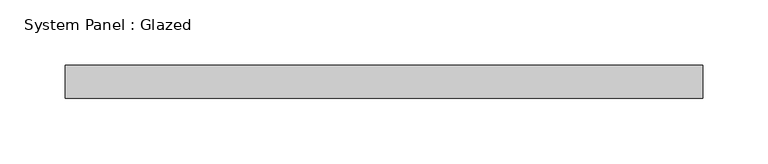
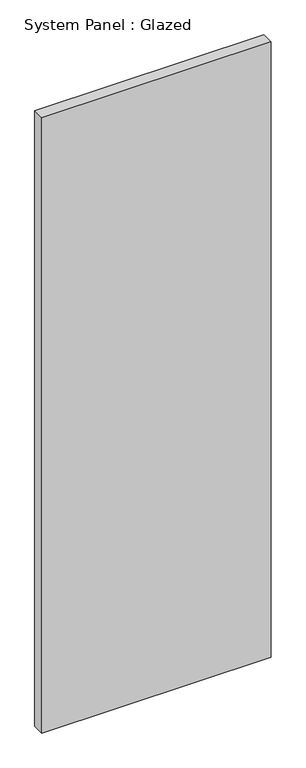
"""IFC4 building model written with IfcOpenShell, lengths in millimetres: plate geometry, System Panel : Glazed."""

from ifc_helpers import new_model, si_unit, origin, origin_with_axes, place, context, project, spatial, polyline, outline, extrude, source, transform, mapped, element, save


def system_panel_glazed_97e07e6e(model_context):
    return source(origin(), model_context, "Body", "SweptSolid", [
        extrude(outline(polyline([(244.475, 19.05), (-244.475, 19.05), (-244.475, 44.45), (244.475, 44.45), (244.475, 19.05)])), origin_with_axes(), (0.0, 0.0, 1.0), 1385.8617517),
    ])


if __name__ == "__main__":
    model = new_model("IFC4")
    model_context = context("Model", 3, world=origin())
    ifc_project = project(units=[si_unit("LENGTHUNIT", "METRE", prefix="MILLI")], contexts=[model_context])
    site = spatial("IfcSite", under=ifc_project)
    building = spatial("IfcBuilding", under=site)
    placement = place(None, origin())
    system_panel_glazed_shape = system_panel_glazed_97e07e6e(model_context)
    element("IfcPlate", 1, ObjectType="System Panel : Glazed", at=placement, inside=building, context=model_context, shape_type="MappedRepresentation", body=[
        mapped(system_panel_glazed_shape, transform((0.0, 0.0, 0.0), x_axis=(1.0, 0.0, 0.0), y_axis=(0.0, 1.0, 0.0), z_axis=(0.0, 0.0, 1.0))),
    ])
    save(model, "model.ifc")

# Revit data of these elements
# Type "System Panel : Glazed"
#   Construction Type Id = "GSP4R"
#   Analytic Construction = "1/8 in Pilkington single glazing"
#   Visual Light Transmittance = 0.9
#   Solar Heat Gain Coefficient = 0.86
#   Heat Transfer Coefficient (U) = 1.18115 BTU/(h·ft²·°F)
#   Define Thermal Properties by = 1
# Element 1 (IfcPlate, "System Panel : Glazed")
#   Materials on its faces: "Glass"
# Materials
#   "Glass": class "Glass", colour RGB 0 128 192, transparency 0.75, Description = "Soda Lime Glass", Cost = 0
